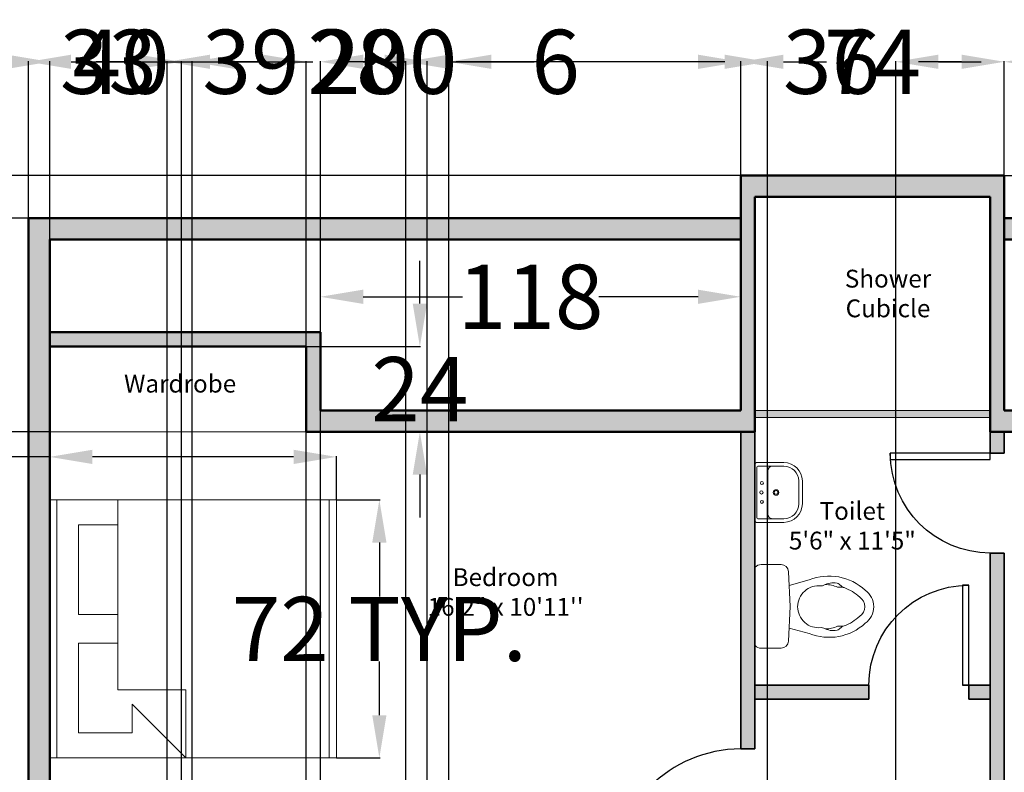
# Model space of a CAD drawing. Units: inches. Extents: x 2 to 695, y -374 to 352.
# Tile 5 of 6: x 144 to 421, y 141 to 352. Entities that reach past the tile are written whole.
import ezdxf

# ---------------------------------------------------------------- set-up
doc = ezdxf.new("R2010")
doc.units = ezdxf.units.IN
for name, color, linetype, lineweight in [('A-ANNO-DIMS', 2, 'Continuous', 18), ('A-ANNO-TEXT', 7, 'Continuous', 18), ('A-AREA-IDEN', 7, 'Continuous', 18), ('A-DOOR', 3, 'Continuous', 25), ('A-FLOR-FIXT', 9, 'Continuous', 18), ('A-WALL-PATT', 252, 'Continuous', 13), ('Furniture', 2, 'Continuous', 18), ('Inner Wall', 5, 'Continuous', 35), ('Outer Wall', 1, 'Continuous', 50)]:
    doc.layers.add(name, color=color, linetype=linetype, lineweight=lineweight)
doc.styles.get("Standard").update_dxf_attribs({"font": 'arial.ttf'})
doc.dimstyles.get("Standard").update_dxf_attribs({"dimtxt": 18, "dimasz": 12, "dimexe": 0.18, "dimexo": 0.0625, "dimgap": 0.09, "dimtad": 0, "dimtih": 1, "dimtoh": 1, "dimdec": 0, "dimzin": 0, "dimdsep": 46, "dimlunit": 3, "dimtxsty": 'Standard', "dimcen": 0.09, "dimadec": 0, "dimazin": 0, "dimtfac": 1, "dimtdec": 0, "dimtofl": 0, "dimtmove": 0, "dimatfit": 3, "dimfxl": 1, "dimtolj": 1, "dimtzin": 0, "dimarcsym": 0})

# ---------------------------------------------------------------- blocks, each defined once
blk = doc.blocks.new('*U2')
for p, q in [((0, 0), (0, -4)), ((36, 0), (36, -4))]:
    blk.add_line(p, q)
blk.add_lwpolyline([(0, 0), (0, 36), (1.75, 36), (1.75, 0)], close=True)
blk.add_arc((0, 0), 36, 0, 90)
blk = doc.blocks.new('*U3')
for p, q in [((0, 0), (0, -4)), ((28, 0), (28, -4))]:
    blk.add_line(p, q)
blk.add_lwpolyline([(0, 0), (0, 28), (1.75, 28), (1.75, 0)], close=True)
blk.add_arc((0, 0), 28, 0, 90)
blk = doc.blocks.new('A$C1308471B')
at = {"ltscale": 20}
for p, q in [((0, 0.4607), (0, 0.0186)), ((0.0354, 0.4793), (0.1495, 0.4793)), ((0.2013, 0.2397), (0.1923, 0.4384)), ((0.1957, 0.3639), (0.3109, 0.3953)), ((0.5021, 0.3528), (0.4724, 0.3528)), ((0.4982, 0.3575), (0.4822, 0.3709)), ((0.2013, 0.2397), (0.1923, 0.0409)), ((0.1959, 0.1193), (0.3109, 0.0879)), ((0.5021, 0.1304), (0.4724, 0.1304)), ((0.4982, 0.1257), (0.4822, 0.1123)), ((0.0354, 0), (0.1495, 0))]:
    blk.add_line(p, q, dxfattribs=at)
for centre, radius, start, end in [((0.006, 0.4607), 0.006, 136.5269, 180), ((0.0354, 0.4328), 0.0465, 90, 136.5269), ((0.1495, 0.4365), 0.0429, 2.5755, 90), ((0.4248, 0.1104), 0.3068, 47.4135, 111.7924), ((0.3654, 0.2416), 0.1206, 83.3523, 180), ((0.3823, 0.3868), 0.0255, 263.3523, 298.5742), ((0.4494, 0.2636), 0.1148, 79.3968, 118.5742), ((0.405, 0.2159), 0.153, 63.502, 90.4522), ((0.4658, 0.3513), 0.0255, 50, 79.3968), ((0.5146, 0.377), 0.0255, 230, 251.3881), ((0.5021, 0.3273), 0.0255, 70.3751, 90), ((0.4248, 0.1104), 0.2558, 46.612, 70.3751), ((0.5654, 0.2416), 0.065, 0, 57.2974), ((0.5654, 0.2416), 0.116, 0, 54.7115), ((0.3654, 0.2416), 0.1206, 180, 276.6477), ((0.5654, 0.2416), 0.065, 302.7026, 0), ((0.5654, 0.2416), 0.116, 305.2885, 0), ((0.4248, 0.3728), 0.2558, 289.6249, 313.388), ((0.4248, 0.3728), 0.3068, 248.2076, 312.5865), ((0.3823, 0.0964), 0.0255, 61.4258, 96.6477), ((0.4494, 0.2196), 0.1148, 241.4258, 280.6032), ((0.405, 0.2673), 0.153, 269.5478, 296.498), ((0.5146, 0.1062), 0.0255, 108.6119, 130), ((0.5021, 0.1559), 0.0255, 270, 289.6249), ((0.4658, 0.1319), 0.0255, 280.6032, 310), ((0.006, 0.0186), 0.006, 180, 223.4731), ((0.0354, 0.0465), 0.0465, 223.4731, 270), ((0.1495, 0.0429), 0.0429, 270, 357.4245)]:
    blk.add_arc(centre, radius, start, end, dxfattribs=at)
blk = doc.blocks.new('A$C57EA129C')
for p, q in [((0, 0.4428), (0, 0.1782)), ((0.016, 0.4589), (0.5631, 0.4589)), ((0.0356, 0.4321), (0.0356, 0.2896)), ((0.0445, 0.441), (0.5346, 0.441)), ((0.5435, 0.4321), (0.5435, 0.2896)), ((0.5791, 0.4428), (0.5791, 0.1782)), ((0.0356, 0.2896), (0.0356, 0.1782)), ((0.0802, 0.3341), (0.499, 0.3341)), ((0.5435, 0.2896), (0.5435, 0.1782)), ((0.1782, 0.0356), (0.4009, 0.0356)), ((0.1782, 0), (0.4009, 0))]:
    blk.add_line(p, q)
for centre, radius in [((0.1982, 0.392), 0.0143), ((0.2896, 0.3965), 0.0156), ((0.3809, 0.392), 0.0143), ((0.2896, 0.2545), 0.0267), ((0.2896, 0.2545), 0.0178)]:
    blk.add_circle(centre, radius)
for centre, radius, start, end in [((0.016, 0.4428), 0.016, 90, 180), ((0.0445, 0.4321), 0.00891, 90, 180), ((0.5346, 0.4321), 0.00891, 0, 90), ((0.5631, 0.4428), 0.016, 0, 90), ((0.0802, 0.2896), 0.0445, 90, 180), ((0.499, 0.2896), 0.0445, 0, 90), ((0.1782, 0.1782), 0.1782, 180, 270), ((0.1782, 0.1782), 0.1426, 180, 270), ((0.4009, 0.1782), 0.1782, 270, 0), ((0.4009, 0.1782), 0.1426, 270, 0)]:
    blk.add_arc(centre, radius, start, end)
blk = doc.blocks.new('KING-00')
for p, q in [((-0.8967, -0.947), (-0.8967, 0.8818)), ((0.6019, 0.8818), (0.6019, -0.4644)), ((1.0337, -0.947), (1.0337, 0.8818)), ((0.6019, 0.704), (0.8813, 0.704)), ((0.8813, 0.069), (0.8813, 0.704)), ((0.6019, 0.069), (0.8813, 0.069)), ((0.8813, -0.1342), (0.6019, -0.1342)), ((0.8813, -0.7692), (0.8813, -0.1342)), ((0.1193, -0.4644), (0.1193, -0.947)), ((0.6019, -0.4644), (0.1193, -0.4644)), ((0.1193, -0.947), (0.5003, -0.566)), ((0.5003, -0.7692), (0.5003, -0.566)), ((0.5003, -0.7692), (0.8813, -0.7692))]:
    blk.add_line(p, q)
blk.add_lwpolyline([(-0.9475, -0.947), (-0.9475, 0.8818), (1.0845, 0.8818), (1.0845, -0.947)], close=True)
blk = doc.blocks.new('*D16')
at = {"layer": 'A-ANNO-DIMS', "color": 0, "lineweight": -2, "transparency": 16777216}
for p, q in [((152.79, 229.15), (140.79, 229.15)), ((152.79, 217.14), (152.79, 229.33)), ((221.26, 229.15), (164.79, 229.15)), ((233.26, 217.14), (233.26, 229.33))]:
    blk.add_line(p, q, dxfattribs=at)
at = {"layer": 'A-ANNO-DIMS', "color": 0, "transparency": 16777216}
for points in [[(164.79, 231.15), (164.79, 227.15), (152.79, 229.15)], [(221.26, 231.15), (221.26, 227.15), (233.26, 229.15)]]:
    blk.add_solid(points, dxfattribs=at)
at = {"layer": 'Defpoints', "color": 0, "transparency": 16777216}
for p in [(152.79, 229.15), (152.79, 217.08), (233.26, 217.08)]:
    blk.add_point(p, dxfattribs=at)
at = {"layer": 'A-ANNO-DIMS', "color": 0, "transparency": 16777216, "insert": (67.94, 229.15), "char_height": 18, "attachment_point": 5}
blk.add_mtext('\\A1;BED 80 TYP.', dxfattribs=at)
blk = doc.blocks.new('*D17')
at = {"layer": 'A-ANNO-DIMS', "color": 0, "lineweight": -2, "transparency": 16777216}
for p, q in [((233.32, 217.08), (245.51, 217.08)), ((245.33, 205.08), (245.33, 190)), ((245.33, 156.66), (245.33, 171.74)), ((233.32, 144.66), (245.51, 144.66))]:
    blk.add_line(p, q, dxfattribs=at)
at = {"layer": 'A-ANNO-DIMS', "color": 0, "transparency": 16777216}
for points in [[(243.33, 205.08), (247.33, 205.08), (245.33, 217.08)], [(243.33, 156.66), (247.33, 156.66), (245.33, 144.66)]]:
    blk.add_solid(points, dxfattribs=at)
at = {"layer": 'Defpoints', "color": 0, "transparency": 16777216}
for p in [(233.26, 217.08), (245.33, 217.08), (233.26, 144.66)]:
    blk.add_point(p, dxfattribs=at)
at = {"layer": 'A-ANNO-DIMS', "color": 0, "transparency": 16777216, "insert": (245.33, 180.87), "char_height": 18, "attachment_point": 5}
blk.add_mtext('\\A1;72 TYP.', dxfattribs=at)
blk = doc.blocks.new('*D29')
at = {"layer": 'A-ANNO-DIMS', "color": 0, "lineweight": -2, "transparency": 16777216}
for p, q in [((420.85, 308.13), (591.88, 308.13)), ((591.7, 296.13), (591.7, -1.56)), ((591.7, -317.82), (591.7, -20.13)), ((217.35, -329.82), (591.88, -329.82))]:
    blk.add_line(p, q, dxfattribs=at)
at = {"layer": 'A-ANNO-DIMS', "color": 0, "transparency": 16777216}
for points in [[(589.7, 296.13), (593.7, 296.13), (591.7, 308.13)], [(589.7, -317.82), (593.7, -317.82), (591.7, -329.82)]]:
    blk.add_solid(points, dxfattribs=at)
at = {"layer": 'Defpoints', "color": 0, "transparency": 16777216}
for p in [(420.79, 308.13), (591.7, 308.13), (217.29, -329.82)]:
    blk.add_point(p, dxfattribs=at)
at = {"layer": 'A-ANNO-DIMS', "color": 0, "transparency": 16777216, "insert": (591.7, -10.85), "char_height": 18, "attachment_point": 5}
blk.add_mtext('\\A1;638', dxfattribs=at)
blk = doc.blocks.new('*D30')
at = {"layer": 'A-ANNO-DIMS', "color": 0, "lineweight": -2, "transparency": 16777216}
for p, q in [((146.79, 296.24), (146.79, 340.22)), ((158.79, 340.04), (226.69, 340.04)), ((334.79, 340.04), (266.88, 340.04)), ((346.79, 308.19), (346.79, 340.22))]:
    blk.add_line(p, q, dxfattribs=at)
at = {"layer": 'A-ANNO-DIMS', "color": 0, "transparency": 16777216}
for points in [[(158.79, 342.04), (158.79, 338.04), (146.79, 340.04)], [(334.79, 342.04), (334.79, 338.04), (346.79, 340.04)]]:
    blk.add_solid(points, dxfattribs=at)
at = {"layer": 'Defpoints', "color": 0, "transparency": 16777216}
for p in [(346.79, 340.04), (346.79, 308.13), (146.79, 296.18)]:
    blk.add_point(p, dxfattribs=at)
at = {"layer": 'A-ANNO-DIMS', "color": 0, "transparency": 16777216, "insert": (246.79, 340.04), "char_height": 18, "attachment_point": 5}
blk.add_mtext('\\A1;200', dxfattribs=at)
blk = doc.blocks.new('*D31')
at = {"layer": 'A-ANNO-DIMS', "color": 0, "lineweight": -2, "transparency": 16777216}
for p, q in [((346.79, 308.19), (346.79, 340.22)), ((358.79, 340.04), (370.91, 340.04)), ((408.79, 340.04), (396.66, 340.04)), ((420.79, 308.19), (420.79, 340.22))]:
    blk.add_line(p, q, dxfattribs=at)
at = {"layer": 'A-ANNO-DIMS', "color": 0, "transparency": 16777216}
for points in [[(358.79, 342.04), (358.79, 338.04), (346.79, 340.04)], [(408.79, 342.04), (408.79, 338.04), (420.79, 340.04)]]:
    blk.add_solid(points, dxfattribs=at)
at = {"layer": 'Defpoints', "color": 0, "transparency": 16777216}
for p in [(420.79, 340.04), (346.79, 308.13), (420.79, 308.13)]:
    blk.add_point(p, dxfattribs=at)
at = {"layer": 'A-ANNO-DIMS', "color": 0, "transparency": 16777216, "insert": (383.79, 340.04), "char_height": 18, "attachment_point": 5}
blk.add_mtext('\\A1;74', dxfattribs=at)
blk = doc.blocks.new('*D32')
at = {"layer": 'A-ANNO-DIMS', "color": 0, "lineweight": -2, "transparency": 16777216}
for p, q in [((420.79, 308.19), (420.79, 340.22)), ((432.79, 340.04), (471.14, 340.04)), ((547.79, 340.04), (509.43, 340.04)), ((559.79, 296.24), (559.79, 340.22))]:
    blk.add_line(p, q, dxfattribs=at)
at = {"layer": 'A-ANNO-DIMS', "color": 0, "transparency": 16777216}
for points in [[(432.79, 342.04), (432.79, 338.04), (420.79, 340.04)], [(547.79, 342.04), (547.79, 338.04), (559.79, 340.04)]]:
    blk.add_solid(points, dxfattribs=at)
at = {"layer": 'Defpoints', "color": 0, "transparency": 16777216}
for p in [(559.79, 340.04), (420.79, 308.13), (559.79, 296.18)]:
    blk.add_point(p, dxfattribs=at)
at = {"layer": 'A-ANNO-DIMS', "color": 0, "transparency": 16777216, "insert": (490.29, 340.04), "char_height": 18, "attachment_point": 5}
blk.add_mtext('\\A1;139', dxfattribs=at)
blk = doc.blocks.new('*D33')
at = {"layer": 'A-ANNO-DIMS', "color": 0, "lineweight": -2, "transparency": 16777216}
for p, q in [((114.87, 320.13), (114.87, 332.13)), ((346.72, 308.13), (114.69, 308.13)), ((146.72, 296.18), (114.69, 296.18)), ((114.87, 284.18), (114.87, 272.18)), ((114.87, 272.18), (102.87, 272.18))]:
    blk.add_line(p, q, dxfattribs=at)
at = {"layer": 'A-ANNO-DIMS', "color": 0, "transparency": 16777216}
for points in [[(112.87, 320.13), (116.87, 320.13), (114.87, 308.13)], [(112.87, 284.18), (116.87, 284.18), (114.87, 296.18)]]:
    blk.add_solid(points, dxfattribs=at)
at = {"layer": 'Defpoints', "color": 0, "transparency": 16777216}
for p in [(346.79, 308.13), (114.87, 296.18), (146.79, 296.18)]:
    blk.add_point(p, dxfattribs=at)
at = {"layer": 'A-ANNO-DIMS', "color": 0, "transparency": 16777216, "insert": (66.2, 272.18), "char_height": 18, "attachment_point": 5}
blk.add_mtext('\\A1;11.955', dxfattribs=at)
blk = doc.blocks.new('*D34')
at = {"layer": 'A-ANNO-DIMS', "color": 0, "lineweight": -2, "transparency": 16777216}
for p, q in [((146.72, 296.18), (114.69, 296.18)), ((114.87, 284.18), (114.87, 275.46)), ((114.87, 248.18), (114.87, 256.89)), ((152.72, 236.18), (114.69, 236.18))]:
    blk.add_line(p, q, dxfattribs=at)
at = {"layer": 'A-ANNO-DIMS', "color": 0, "transparency": 16777216}
for points in [[(112.87, 284.18), (116.87, 284.18), (114.87, 296.18)], [(112.87, 248.18), (116.87, 248.18), (114.87, 236.18)]]:
    blk.add_solid(points, dxfattribs=at)
at = {"layer": 'Defpoints', "color": 0, "transparency": 16777216}
for p in [(146.79, 296.18), (114.87, 236.18), (152.79, 236.18)]:
    blk.add_point(p, dxfattribs=at)
at = {"layer": 'A-ANNO-DIMS', "color": 0, "transparency": 16777216, "insert": (114.87, 266.18), "char_height": 18, "attachment_point": 5}
blk.add_mtext('\\A1;60', dxfattribs=at)
blk = doc.blocks.new('*D39')
at = {"layer": 'A-ANNO-DIMS', "color": 0, "lineweight": -2, "transparency": 16777216}
for p, q in [((212.785845, 340.044756), (200.785845, 340.044756)), ((224.785845, 101.237546), (224.785845, 340.224756)), ((252.785845, 101.237546), (252.785845, 340.224756)), ((264.785845, 340.044756), (276.785845, 340.044756))]:
    blk.add_line(p, q, dxfattribs=at)
at = {"layer": 'A-ANNO-DIMS', "color": 0, "transparency": 16777216}
for points in [[(212.785845, 342.044756), (212.785845, 338.044756), (224.785845, 340.044756)], [(264.785845, 342.044756), (264.785845, 338.044756), (252.785845, 340.044756)]]:
    blk.add_solid(points, dxfattribs=at)
at = {"layer": 'Defpoints', "color": 0, "transparency": 16777216}
for p in [(252.785845, 340.044756), (224.785845, 101.175046), (252.785845, 101.175046)]:
    blk.add_point(p, dxfattribs=at)
at = {"layer": 'A-ANNO-DIMS', "color": 0, "transparency": 16777216, "insert": (238.785845, 340.044756), "char_height": 18, "attachment_point": 5}
blk.add_mtext('\\A1;28', dxfattribs=at)
blk = doc.blocks.new('*D40')
at = {"layer": 'A-ANNO-DIMS', "color": 0, "lineweight": -2, "transparency": 16777216}
for p, q in [((140.785845, 340.044756), (128.785845, 340.044756)), ((152.785845, 101.237546), (152.785845, 340.224756)), ((192.785845, 101.237546), (192.785845, 340.224756)), ((204.785845, 340.044756), (216.785845, 340.044756))]:
    blk.add_line(p, q, dxfattribs=at)
at = {"layer": 'A-ANNO-DIMS', "color": 0, "transparency": 16777216}
for points in [[(140.785845, 342.044756), (140.785845, 338.044756), (152.785845, 340.044756)], [(204.785845, 342.044756), (204.785845, 338.044756), (192.785845, 340.044756)]]:
    blk.add_solid(points, dxfattribs=at)
at = {"layer": 'Defpoints', "color": 0, "transparency": 16777216}
for p in [(192.785845, 340.044756), (152.785845, 101.175046), (192.785845, 101.175046)]:
    blk.add_point(p, dxfattribs=at)
at = {"layer": 'A-ANNO-DIMS', "color": 0, "transparency": 16777216, "insert": (172.785845, 340.044756), "char_height": 18, "attachment_point": 5}
blk.add_mtext('\\A1;40', dxfattribs=at)
blk = doc.blocks.new('*D41')
at = {"layer": 'A-ANNO-DIMS', "color": 0, "lineweight": -2, "transparency": 16777216}
for p, q in [((342.285845, 340.044756), (330.285845, 340.044756)), ((354.285845, -164.762454), (354.285845, 340.224756)), ((390.285845, -164.762454), (390.285845, 340.224756)), ((402.285845, 340.044756), (414.285845, 340.044756))]:
    blk.add_line(p, q, dxfattribs=at)
at = {"layer": 'A-ANNO-DIMS', "color": 0, "transparency": 16777216}
for points in [[(342.285845, 342.044756), (342.285845, 338.044756), (354.285845, 340.044756)], [(402.285845, 342.044756), (402.285845, 338.044756), (390.285845, 340.044756)]]:
    blk.add_solid(points, dxfattribs=at)
at = {"layer": 'Defpoints', "color": 0, "transparency": 16777216}
for p in [(390.285845, 340.044756), (354.285845, -164.824954), (390.285845, -164.824954)]:
    blk.add_point(p, dxfattribs=at)
at = {"layer": 'A-ANNO-DIMS', "color": 0, "transparency": 16777216, "insert": (372.285845, 340.044756), "char_height": 18, "attachment_point": 5}
blk.add_mtext('\\A1;36', dxfattribs=at)
blk = doc.blocks.new('*D45')
at = {"layer": 'A-ANNO-DIMS', "color": 0, "lineweight": -2, "transparency": 16777216}
for p, q in [((246.79, 340.04), (234.79, 340.04)), ((258.79, 105.24), (258.79, 340.22)), ((264.79, 105.24), (264.79, 340.22)), ((276.79, 340.04), (288.79, 340.04))]:
    blk.add_line(p, q, dxfattribs=at)
at = {"layer": 'A-ANNO-DIMS', "color": 0, "transparency": 16777216}
for points in [[(246.79, 342.04), (246.79, 338.04), (258.79, 340.04)], [(276.79, 342.04), (276.79, 338.04), (264.79, 340.04)]]:
    blk.add_solid(points, dxfattribs=at)
at = {"layer": 'Defpoints', "color": 0, "transparency": 16777216}
for p in [(264.79, 340.04), (258.79, 105.18), (264.79, 105.18)]:
    blk.add_point(p, dxfattribs=at)
at = {"layer": 'A-ANNO-DIMS', "color": 0, "transparency": 16777216, "insert": (294.82, 340.04), "char_height": 18, "attachment_point": 5}
blk.add_mtext('\\A1;6', dxfattribs=at)
blk = doc.blocks.new('*D46')
at = {"layer": 'A-ANNO-DIMS', "color": 0, "lineweight": -2, "transparency": 16777216}
for p, q in [((140.785845, 340.044756), (128.785845, 340.044756)), ((152.785845, -48.762454), (152.785845, 340.224756)), ((185.785845, -48.762454), (185.785845, 340.224756)), ((197.785845, 340.044756), (209.785845, 340.044756))]:
    blk.add_line(p, q, dxfattribs=at)
at = {"layer": 'A-ANNO-DIMS', "color": 0, "transparency": 16777216}
for points in [[(140.785845, 342.044756), (140.785845, 338.044756), (152.785845, 340.044756)], [(197.785845, 342.044756), (197.785845, 338.044756), (185.785845, 340.044756)]]:
    blk.add_solid(points, dxfattribs=at)
at = {"layer": 'Defpoints', "color": 0, "transparency": 16777216}
for p in [(185.785845, 340.044756), (152.785845, -48.824954), (185.785845, -48.824954)]:
    blk.add_point(p, dxfattribs=at)
at = {"layer": 'A-ANNO-DIMS', "color": 0, "transparency": 16777216, "insert": (169.285845, 340.044756), "char_height": 18, "attachment_point": 5}
blk.add_mtext('\\A1;33', dxfattribs=at)
blk = doc.blocks.new('*D47')
at = {"layer": 'A-ANNO-DIMS', "color": 0, "lineweight": -2, "transparency": 16777216}
for p, q in [((177.785845, 340.044756), (165.785845, 340.044756)), ((189.785845, -48.762454), (189.785845, 340.224756)), ((228.785845, -48.762454), (228.785845, 340.224756)), ((240.785845, 340.044756), (252.785845, 340.044756))]:
    blk.add_line(p, q, dxfattribs=at)
at = {"layer": 'A-ANNO-DIMS', "color": 0, "transparency": 16777216}
for points in [[(177.785845, 342.044756), (177.785845, 338.044756), (189.785845, 340.044756)], [(240.785845, 342.044756), (240.785845, 338.044756), (228.785845, 340.044756)]]:
    blk.add_solid(points, dxfattribs=at)
at = {"layer": 'Defpoints', "color": 0, "transparency": 16777216}
for p in [(228.785845, 340.044756), (189.785845, -48.824954), (228.785845, -48.824954)]:
    blk.add_point(p, dxfattribs=at)
at = {"layer": 'A-ANNO-DIMS', "color": 0, "transparency": 16777216, "insert": (209.285845, 340.044756), "char_height": 18, "attachment_point": 5}
blk.add_mtext('\\A1;39', dxfattribs=at)
blk = doc.blocks.new('*D53')
at = {"layer": 'A-ANNO-DIMS', "color": 0, "lineweight": -2, "transparency": 16777216}
for p, q in [((228.79, 242.24), (228.79, 274.27)), ((240.79, 274.09), (268.64, 274.09)), ((334.79, 274.09), (306.93, 274.09)), ((346.79, 242.24), (346.79, 274.27))]:
    blk.add_line(p, q, dxfattribs=at)
at = {"layer": 'A-ANNO-DIMS', "color": 0, "transparency": 16777216}
for points in [[(240.79, 276.09), (240.79, 272.09), (228.79, 274.09)], [(334.79, 276.09), (334.79, 272.09), (346.79, 274.09)]]:
    blk.add_solid(points, dxfattribs=at)
at = {"layer": 'Defpoints', "color": 0, "transparency": 16777216}
for p in [(346.79, 274.09), (228.79, 242.18), (346.79, 242.18)]:
    blk.add_point(p, dxfattribs=at)
at = {"layer": 'A-ANNO-DIMS', "color": 0, "transparency": 16777216, "insert": (287.79, 274.09), "char_height": 18, "attachment_point": 5}
blk.add_mtext('\\A1;118', dxfattribs=at)
blk = doc.blocks.new('*D54')
at = {"layer": 'A-ANNO-DIMS', "color": 0, "lineweight": -2, "transparency": 16777216}
for p, q in [((256.700845, 272.175046), (256.700845, 284.175046)), ((224.848345, 260.175046), (256.880845, 260.175046)), ((224.848345, 236.175046), (256.880845, 236.175046)), ((256.700845, 224.175046), (256.700845, 212.175046))]:
    blk.add_line(p, q, dxfattribs=at)
at = {"layer": 'A-ANNO-DIMS', "color": 0, "transparency": 16777216}
for points in [[(254.700845, 272.175046), (258.700845, 272.175046), (256.700845, 260.175046)], [(254.700845, 224.175046), (258.700845, 224.175046), (256.700845, 236.175046)]]:
    blk.add_solid(points, dxfattribs=at)
at = {"layer": 'Defpoints', "color": 0, "transparency": 16777216}
for p in [(224.785845, 260.175046), (224.785845, 236.175046), (256.700845, 236.175046)]:
    blk.add_point(p, dxfattribs=at)
at = {"layer": 'A-ANNO-DIMS', "color": 0, "transparency": 16777216, "insert": (256.700845, 248.175046), "char_height": 18, "attachment_point": 5}
blk.add_mtext('\\A1;24', dxfattribs=at)

msp = doc.modelspace()

# ---------------------------------------------------------------- hatches: boundary and pattern name
at = {"layer": 'A-WALL-PATT'}
h = msp.add_hatch(color=256, dxfattribs=at)
h.dxf.hatch_style = 1
h.paths.add_polyline_path([(346.7858, 296.175), (146.7858, 296.175), (146.7858, -329.825), (217.2858, -329.825), (217.2858, -305.825), (559.7858, -305.825), (559.7858, 296.175), (420.7858, 296.175), (420.7858, 290.175), (553.7858, 290.175), (553.7858, -299.825), (213.2858, -299.825), (213.2858, -323.825), (152.7858, -323.825), (152.7858, 290.175), (346.7858, 290.175)])
h.paths.add_polyline_path([(420.7858, 308.1298), (346.7858, 308.1298), (346.7858, 242.175), (228.7858, 242.175), (228.7858, 264.175), (152.7858, 264.175), (152.7858, 260.175), (224.7858, 260.175), (224.7858, 236.175), (350.7858, 236.175), (350.7858, 302.1298), (416.7858, 302.1298), (416.7858, 236.175), (553.7858, 236.175), (553.7858, 242.175), (420.7858, 242.175)])
h = msp.add_hatch(color=256, dxfattribs=at)
h.dxf.hatch_style = 1
h.paths.add_polyline_path([(394.2858, -160.825), (390.2858, -160.825), (390.2858, -164.825), (390.2858, -299.825), (394.2858, -299.825)])
h.paths.add_polyline_path([(217.2858, -235.1253), (213.2858, -235.1253), (213.2858, -299.825), (217.2858, -299.825)])
h.paths.add_polyline_path([(213.2858, -273.825), (152.7858, -273.825), (152.7858, -275.825), (213.2858, -275.825)])
h.paths.add_polyline_path([(354.2858, -160.825), (350.7858, -160.825), (350.7858, -124.825), (346.7858, -124.825), (346.7858, -160.825), (152.7858, -160.825), (152.7858, -164.825), (213.2858, -164.825), (213.2858, -188.8137), (213.2858, -207.1253), (217.2858, -207.1253), (217.2858, -187.1253), (217.2858, -164.825), (354.2858, -164.825)])
h.paths.add_polyline_path([(350.7858, -20.825), (346.7858, -20.825), (346.7858, -48.825), (152.7858, -48.825), (152.7858, -52.825), (249.7858, -52.825), (346.7858, -52.825), (346.7858, -88.825), (350.7858, -88.825)])
h.paths.add_polyline_path([(189.7858, 33.175), (185.7858, 33.175), (185.7858, -48.825), (189.7858, -48.825)])
h.paths.add_polyline_path([(334.7858, 37.175), (264.7858, 37.175), (264.7858, 33.175), (334.7858, 33.175)])
h.paths.add_polyline_path([(258.7858, 37.175), (152.7858, 37.175), (152.7858, 33.175), (258.7858, 33.175)])
h.paths.add_polyline_path([(194.7858, 101.175), (192.7858, 101.175), (192.7858, 37.175), (194.7858, 37.175)])
h.paths.add_polyline_path([(264.7858, 105.175), (258.7858, 105.175), (258.7858, 33.175), (264.7858, 33.175), (264.7858, 37.175)])
h.paths.add_polyline_path([(340.7858, 105.175), (334.7858, 105.175), (334.7858, 33.175), (340.7858, 33.175)])
h.paths.add_polyline_path([(350.7858, 111.175), (346.7858, 111.175), (346.7858, 105.175), (340.7858, 105.175), (340.7858, 101.175), (350.7858, 101.175)])
h.paths.add_polyline_path([(350.7858, 37.175), (340.7858, 37.175), (340.7858, 33.175), (346.7858, 33.175), (346.7858, 27.175), (350.7858, 27.175)])
h.paths.add_polyline_path([(334.7858, 105.175), (264.7858, 105.175), (264.7858, 101.175), (334.7858, 101.175)])
h.paths.add_polyline_path([(258.7858, 105.175), (252.7858, 105.175), (252.7858, 101.175), (258.7858, 101.175)])
h.paths.add_polyline_path([(224.7858, 105.175), (152.7858, 105.175), (152.7858, 101.175), (224.7858, 101.175)])
h.paths.add_polyline_path([(382.7858, 165.1298), (350.7858, 165.1298), (350.7858, 161.1298), (382.7858, 161.1298)])
h.paths.add_polyline_path([(350.7858, 236.175), (346.7858, 236.175), (346.7858, 147.175), (350.7858, 147.175)])
h.paths.add_polyline_path([(420.7858, 202.175), (416.7858, 202.175), (416.7858, 101.175), (420.7858, 101.175)])
h.paths.add_polyline_path([(416.7858, 165.1298), (410.7858, 165.1298), (410.7858, 161.1298), (416.7858, 161.1298)])
h.paths.add_polyline_path([(416.7858, 242.175), (350.7858, 242.175), (350.7858, 240.175), (416.7858, 240.175)])
h.paths.add_polyline_path([(420.7858, 236.175), (416.7858, 236.175), (416.7858, 230.175), (420.7858, 230.175)])
h.paths.add_polyline_path([(553.7858, 59.175), (469.3071, 59.175), (420.7858, 59.175), (420.7858, 65.175), (416.7858, 65.175), (416.7858, 55.175), (553.7858, 55.175)])

# ---------------------------------------------------------------- linework, layer by layer
at = {"layer": 'A-FLOR-FIXT'}
for p, q in [((350.7858, 242.175), (416.7858, 242.175)), ((350.7858, 240.175), (416.7858, 240.175))]:
    msp.add_line(p, q, dxfattribs=at)
at = {"layer": 'Furniture'}
msp.add_lwpolyline([(152.7858, 260.175), (224.7858, 260.175), (224.7858, 236.175), (152.7858, 236.175)], close=True, dxfattribs=at)
at = {"layer": 'Inner Wall'}
for p, q in [((346.7858, 147.175), (346.7858, 236.175)), ((350.7858, 236.175), (350.7858, 147.175)), ((416.7858, 230.175), (416.7858, 236.175)), ((420.7858, 230.175), (420.7858, 236.175)), ((416.7858, 230.175), (420.7858, 230.175)), ((416.7858, 101.175), (416.7858, 202.175)), ((416.7858, 202.175), (420.7858, 202.175)), ((420.7858, 101.175), (420.7858, 202.175)), ((350.7858, 165.1298), (382.7858, 165.1298)), ((382.7858, 161.1298), (382.7858, 165.1298)), ((409.0358, 165.1298), (416.7858, 165.1298)), ((410.7858, 161.1298), (410.7858, 165.1298)), ((350.7858, 161.1298), (382.7858, 161.1298)), ((410.7858, 161.1298), (416.7858, 161.1298)), ((350.7858, 147.175), (346.7858, 147.175))]:
    msp.add_line(p, q, dxfattribs=at)
at = {"layer": 'Outer Wall'}
for p, q in [((346.7858, 242.175), (346.7858, 308.1298)), ((346.7858, 308.1298), (420.7858, 308.1298)), ((420.7858, 242.175), (420.7858, 308.1298)), ((350.7858, 302.1298), (416.7858, 302.1298)), ((350.7858, 236.175), (350.7858, 302.1298)), ((416.7858, 236.175), (416.7858, 302.1298)), ((146.7858, -329.825), (146.7858, 296.175)), ((146.7858, 296.175), (346.7858, 296.175)), ((559.7858, 296.175), (420.7858, 296.175)), ((152.7858, -323.825), (152.7858, 290.175)), ((152.7858, 290.175), (346.7858, 290.175)), ((553.7858, 290.175), (420.7858, 290.175)), ((152.7858, 264.175), (228.7858, 264.175)), ((228.7858, 242.175), (228.7858, 264.175)), ((152.7858, 260.175), (224.7858, 260.175)), ((224.7858, 236.175), (224.7858, 260.175)), ((228.7858, 242.175), (346.7858, 242.175)), ((420.7858, 242.175), (553.7858, 242.175)), ((224.7858, 236.175), (350.7858, 236.175)), ((416.7858, 236.175), (553.7858, 236.175))]:
    msp.add_line(p, q, dxfattribs=at)

# ---------------------------------------------------------------- block references
at = {"layer": 'A-DOOR', "xscale": -1}
for p, rotation in [((416.7858, 230.175), 89.99999999999991), ((410.7858, 165.1298), 359.9999999999999)]:
    msp.add_blockref('*U3', p, dxfattribs=dict(at, rotation=rotation))
at = {"layer": 'A-DOOR', "rotation": 89.99999999999999}
msp.add_blockref('*U2', (346.7858, 111.175), dxfattribs=at)
at = {"layer": 'A-FLOR-FIXT'}
for name, p, xscale, yscale, zscale, rotation in [('A$C57EA129C', (364.0853, 227.5634), -28.98333223671166, 28.98333223671166, 28.98333223671166, 90), ('A$C1308471B', (350.7858, 198.9291), -48.95497407897215, 48.95497407897215, 48.95497407897215, 180)]:
    msp.add_blockref(name, p, dxfattribs=dict(at, xscale=xscale, yscale=yscale, zscale=zscale, rotation=rotation))
at = {"layer": 'Furniture', "xscale": -39.60249106241186, "yscale": 39.60249106241186, "zscale": 39.60249106241186}
msp.add_blockref('KING-00', (195.7347, 182.1583), dxfattribs=at)

# ---------------------------------------------------------------- texts
at = {"layer": 'A-ANNO-TEXT', "char_height": 5, "attachment_point": 3}
for s, insert in [('\\pxqc;{\\fTimes New Roman|b0|i0|c0|p18;Shower\\PCubicle}', (412.682, 281.6763)), ('\\pxqc;{\\fTimes New Roman|b0|i0|c0|p18;Wardrobe}', (213.9497, 252.2109))]:
    msp.add_mtext_dynamic_manual_height_columns(s, width=49.101878, gutter_width=12.5, heights=[0], dxfattribs=dict(at, insert=insert))
at = {"layer": 'A-AREA-IDEN', "char_height": 5, "attachment_point": 3}
for s, insert in [('\\pxqc;{\\fTimes New Roman|b0|i0|c0|p18;Toilet\\P5\'6" x 11\'5"}', (402.6655, 216.4888)), ('\\pxqc;{\\fTimes New Roman|b0|i0|c0|p18;Bedroom\\P16\'2" x 10\'11\'\'}', (305.3063, 197.8971))]:
    msp.add_mtext_dynamic_manual_height_columns(s, width=49.101878, gutter_width=12.5, heights=[0], dxfattribs=dict(at, insert=insert))

# ---------------------------------------------------------------- dimensions: what is measured, and where the dimension line sits
at = {"layer": 'A-ANNO-DIMS'}
for base, p1, p2, picture, middle in [((192.7858, 340.0448), (152.7858, 101.175), (192.7858, 101.175), '*D40', (172.7858, 340.0448)), ((185.7858, 340.0448), (152.7858, -48.825), (185.7858, -48.825), '*D46', (169.2858, 340.0448)), ((346.7858, 340.0448), (146.7858, 296.175), (346.7858, 308.1298), '*D30', (246.7858, 340.0448)), ((228.7858, 340.0448), (189.7858, -48.825), (228.7858, -48.825), '*D47', (209.2858, 340.0448)), ((252.7858, 340.0448), (224.7858, 101.175), (252.7858, 101.175), '*D39', (238.7858, 340.0448)), ((264.7858, 340.0448), (258.7858, 105.175), (264.7858, 105.175), '*D45', (294.8185, 340.0448)), ((390.2858, 340.0448), (354.2858, -164.825), (390.2858, -164.825), '*D41', (372.2858, 340.0448)), ((420.7858, 340.0448), (346.7858, 308.1298), (420.7858, 308.1298), '*D31', (383.7858, 340.0448)), ((559.7858, 340.0448), (420.7858, 308.1298), (559.7858, 296.175), '*D32', (490.2858, 340.0448))]:
    dim = msp.add_linear_dim(base=base, p1=p1, p2=p2, dimstyle='Standard', override={"dimdec": 0, "dimlfac": 1, "dimrnd": 0, "dimzin": 0, "dimdsep": 46, "dimlunit": 2}, dxfattribs=at)
    dim.commit()
    dim.dimension.update_dxf_attribs({"geometry": picture, "text_midpoint": middle})
for base, p1, p2, angle, override, picture, middle in [((114.8708, 296.175), (346.7858, 308.1298), (146.7858, 296.175), 90, {"dimdec": 3, "dimlfac": 1, "dimrnd": 0, "dimzin": 0, "dimdsep": 46, "dimlunit": 2}, '*D33', (66.1976, 272.175)), ((591.7008, 308.1298), (217.2858, -329.825), (420.7858, 308.1298), 90, {"dimdec": 0, "dimlfac": 1, "dimrnd": 0, "dimzin": 0, "dimdsep": 46, "dimlunit": 2}, '*D29', (591.7008, -10.8476)), ((114.8708, 236.175), (146.7858, 296.175), (152.7858, 236.175), 90, {"dimdec": 0, "dimlfac": 1, "dimrnd": 0, "dimzin": 0, "dimdsep": 46, "dimlunit": 2}, '*D34', (114.8708, 266.175)), ((346.7858, 274.09), (228.7858, 242.175), (346.7858, 242.175), 0, {"dimdec": 0, "dimlfac": 1, "dimrnd": 0, "dimzin": 0, "dimdsep": 46, "dimlunit": 2}, '*D53', (287.7858, 274.09)), ((256.7008, 236.175), (224.7858, 260.175), (224.7858, 236.175), 270, {"dimdec": 0, "dimlfac": 1, "dimrnd": 0, "dimzin": 0, "dimdsep": 46, "dimlunit": 2}, '*D54', (256.7008, 248.175))]:
    dim = msp.add_linear_dim(base=base, p1=p1, p2=p2, angle=angle, dimstyle='Standard', override=override, dxfattribs=at)
    dim.commit()
    dim.dimension.update_dxf_attribs({"geometry": picture, "text_midpoint": middle})
for base, p1, p2, angle, text, picture, middle in [((152.7858, 229.1519), (233.2581, 217.0811), (152.7858, 217.0811), 180, 'BED <> TYP.', '*D16', (67.9407, 229.1519)), ((245.3289, 217.0811), (233.2581, 144.6561), (233.2581, 217.0811), 90, '<> TYP.', '*D17', (245.3289, 180.8686))]:
    dim = msp.add_linear_dim(base=base, p1=p1, p2=p2, angle=angle, text=text, dimstyle='Standard', override={"dimdec": 0, "dimlfac": 1, "dimrnd": 0, "dimzin": 0, "dimdsep": 46, "dimlunit": 2}, dxfattribs=at)
    dim.commit()
    dim.dimension.update_dxf_attribs({"geometry": picture, "text_midpoint": middle})

doc.saveas('drawing.dxf')
